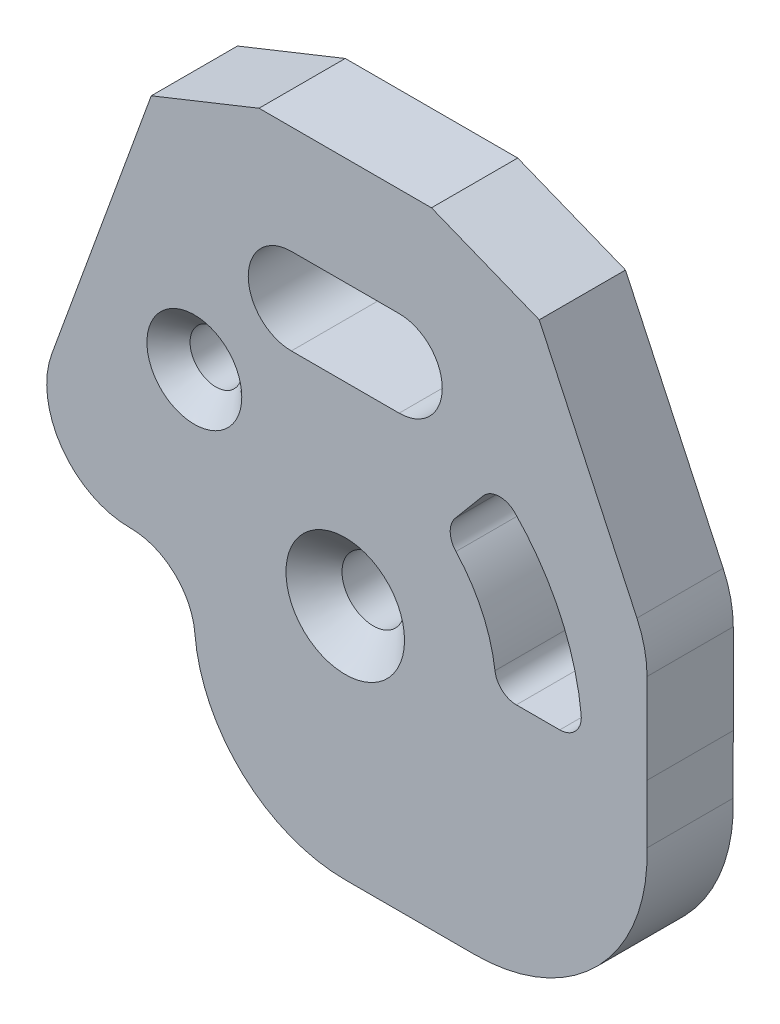
ISO-10303-21;
HEADER;
FILE_DESCRIPTION(('STEP AP214'),'2;1');
FILE_NAME('part.step','',(''),(''),'','','');
FILE_SCHEMA(('AUTOMOTIVE_DESIGN { 1 0 10303 214 1 1 1 1 }'));
ENDSEC;
DATA;
#1=APPLICATION_CONTEXT('core data for automotive mechanical design processes');
#2=APPLICATION_PROTOCOL_DEFINITION('international standard','automotive_design',2000,#1);
#3=PRODUCT_CONTEXT('',#1,'mechanical');
#4=PRODUCT('Part','Part','',(#3));
#5=PRODUCT_RELATED_PRODUCT_CATEGORY('part','',(#4));
#6=PRODUCT_DEFINITION_FORMATION('','',#4);
#7=PRODUCT_DEFINITION_CONTEXT('part definition',#1,'design');
#8=PRODUCT_DEFINITION('design','',#6,#7);
#9=PRODUCT_DEFINITION_SHAPE('','',#8);
#10=(LENGTH_UNIT() NAMED_UNIT(*) SI_UNIT(.MILLI.,.METRE.));
#11=(NAMED_UNIT(*) PLANE_ANGLE_UNIT() SI_UNIT($,.RADIAN.));
#12=(NAMED_UNIT(*) SI_UNIT($,.STERADIAN.) SOLID_ANGLE_UNIT());
#13=UNCERTAINTY_MEASURE_WITH_UNIT(LENGTH_MEASURE(1.E-05),#10,'distance_accuracy_value','');
#14=(GEOMETRIC_REPRESENTATION_CONTEXT(3) GLOBAL_UNCERTAINTY_ASSIGNED_CONTEXT((#13)) GLOBAL_UNIT_ASSIGNED_CONTEXT((#10,
#11,#12)) REPRESENTATION_CONTEXT('',''));
#15=CARTESIAN_POINT('',(0.,0.,0.));
#16=DIRECTION('',(0.,0.,1.));
#17=DIRECTION('',(1.,0.,0.));
#18=AXIS2_PLACEMENT_3D('',#15,#16,#17);
#19=CARTESIAN_POINT('',(-4.,4.47424171782655,4.));
#20=DIRECTION('',(0.371390676354104,-0.928476690885259,0.));
#21=DIRECTION('',(0.928476690885259,0.371390676354104,0.));
#22=AXIS2_PLACEMENT_3D('',#19,#20,#21);
#23=PLANE('',#22);
#24=DIRECTION('',(-0.928476690885259,-0.371390676354104,0.));
#25=VECTOR('',#24,1.);
#26=CARTESIAN_POINT('',(-4.,4.47424171782655,0.));
#27=LINE('',#26,#25);
#28=CARTESIAN_POINT('',(-4.,4.47424171782655,0.));
#29=VERTEX_POINT('',#28);
#30=CARTESIAN_POINT('',(-9.,2.47424171782655,0.));
#31=VERTEX_POINT('',#30);
#32=EDGE_CURVE('E248',#29,#31,#27,.T.);
#33=ORIENTED_EDGE('',*,*,#32,.T.);
#34=DIRECTION('',(0.,0.,-1.));
#35=VECTOR('',#34,1.);
#36=CARTESIAN_POINT('',(-9.,2.47424171782655,4.));
#37=LINE('',#36,#35);
#38=CARTESIAN_POINT('',(-9.,2.47424171782655,4.));
#39=VERTEX_POINT('',#38);
#40=EDGE_CURVE('E11',#39,#31,#37,.T.);
#41=ORIENTED_EDGE('',*,*,#40,.F.);
#42=DIRECTION('',(-0.928476690885259,-0.371390676354104,0.));
#43=VECTOR('',#42,1.);
#44=CARTESIAN_POINT('',(-4.,4.47424171782655,4.));
#45=LINE('',#44,#43);
#46=CARTESIAN_POINT('',(-4.,4.47424171782655,4.));
#47=VERTEX_POINT('',#46);
#48=EDGE_CURVE('E311',#47,#39,#45,.T.);
#49=ORIENTED_EDGE('',*,*,#48,.F.);
#50=DIRECTION('',(0.,0.,-1.));
#51=VECTOR('',#50,1.);
#52=CARTESIAN_POINT('',(-4.,4.47424171782655,4.));
#53=LINE('',#52,#51);
#54=EDGE_CURVE('E343',#47,#29,#53,.T.);
#55=ORIENTED_EDGE('',*,*,#54,.T.);
#56=EDGE_LOOP('',(#33,#41,#49,#55));
#57=FACE_BOUND('',#56,.T.);
#58=ADVANCED_FACE('F39',(#57),#23,.F.);
#59=CARTESIAN_POINT('',(-9.,2.47424171782655,4.));
#60=DIRECTION('',(0.93969262078591,-0.342020143325666,0.));
#61=DIRECTION('',(0.342020143325666,0.93969262078591,0.));
#62=AXIS2_PLACEMENT_3D('',#59,#60,#61);
#63=PLANE('',#62);
#64=DIRECTION('',(-0.342020143325666,-0.93969262078591,0.));
#65=VECTOR('',#64,1.);
#66=CARTESIAN_POINT('',(-9.,2.47424171782655,0.));
#67=LINE('',#66,#65);
#68=CARTESIAN_POINT('',(-13.6164910462462,-10.2094631888496,0.));
#69=VERTEX_POINT('',#68);
#70=EDGE_CURVE('E342',#31,#69,#67,.T.);
#71=ORIENTED_EDGE('',*,*,#70,.T.);
#72=DIRECTION('',(0.,0.,-1.));
#73=VECTOR('',#72,1.);
#74=CARTESIAN_POINT('',(-13.6164910462462,-10.2094631888496,4.));
#75=LINE('',#74,#73);
#76=CARTESIAN_POINT('',(-13.6164910462462,-10.2094631888496,4.));
#77=VERTEX_POINT('',#76);
#78=EDGE_CURVE('E50',#77,#69,#75,.T.);
#79=ORIENTED_EDGE('',*,*,#78,.F.);
#80=DIRECTION('',(-0.342020143325666,-0.93969262078591,0.));
#81=VECTOR('',#80,1.);
#82=CARTESIAN_POINT('',(-9.,2.47424171782655,4.));
#83=LINE('',#82,#81);
#84=EDGE_CURVE('E316',#39,#77,#83,.T.);
#85=ORIENTED_EDGE('',*,*,#84,.F.);
#86=ORIENTED_EDGE('',*,*,#40,.T.);
#87=EDGE_LOOP('',(#71,#79,#85,#86));
#88=FACE_BOUND('',#87,.T.);
#89=ADVANCED_FACE('F439',(#88),#63,.F.);
#90=CARTESIAN_POINT('',(-10.,-11.5257582821734,4.));
#91=DIRECTION('',(0.,0.,-1.));
#92=DIRECTION('',(-1.,0.,0.));
#93=AXIS2_PLACEMENT_3D('',#90,#91,#92);
#94=CYLINDRICAL_SURFACE('',#93,3.84858938577341);
#95=CARTESIAN_POINT('',(-10.,-11.5257582821734,0.));
#96=DIRECTION('',(0.,0.,1.));
#97=DIRECTION('',(1.,0.,0.));
#98=AXIS2_PLACEMENT_3D('',#95,#96,#97);
#99=CIRCLE('',#98,3.84858938577341);
#100=CARTESIAN_POINT('',(-9.97975073778593,-15.3742943970706,0.));
#101=VERTEX_POINT('',#100);
#102=EDGE_CURVE('E347',#69,#101,#99,.T.);
#103=ORIENTED_EDGE('',*,*,#102,.T.);
#104=DIRECTION('',(0.,0.,-1.));
#105=VECTOR('',#104,1.);
#106=CARTESIAN_POINT('',(-9.97975073778593,-15.3742943970706,4.));
#107=LINE('',#106,#105);
#108=CARTESIAN_POINT('',(-9.97975073778593,-15.3742943970706,4.));
#109=VERTEX_POINT('',#108);
#110=EDGE_CURVE('E398',#109,#101,#107,.T.);
#111=ORIENTED_EDGE('',*,*,#110,.F.);
#112=CARTESIAN_POINT('',(-10.,-11.5257582821734,4.));
#113=DIRECTION('',(0.,0.,1.));
#114=DIRECTION('',(1.,0.,0.));
#115=AXIS2_PLACEMENT_3D('',#112,#113,#114);
#116=CIRCLE('',#115,3.84858938577341);
#117=EDGE_CURVE('E317',#77,#109,#116,.T.);
#118=ORIENTED_EDGE('',*,*,#117,.F.);
#119=ORIENTED_EDGE('',*,*,#78,.T.);
#120=EDGE_LOOP('',(#103,#111,#118,#119));
#121=FACE_BOUND('',#120,.T.);
#122=ADVANCED_FACE('F443',(#121),#94,.T.);
#123=CARTESIAN_POINT('',(-9.96396614634065,-18.374283709959,4.));
#124=DIRECTION('',(0.,0.,-1.));
#125=DIRECTION('',(-1.,0.,0.));
#126=AXIS2_PLACEMENT_3D('',#123,#124,#125);
#127=CYLINDRICAL_SURFACE('',#126,3.00003083830351);
#128=CARTESIAN_POINT('',(-9.96396614634065,-18.374283709959,0.));
#129=DIRECTION('',(0.,0.,-1.));
#130=DIRECTION('',(1.,0.,0.));
#131=AXIS2_PLACEMENT_3D('',#128,#129,#130);
#132=CIRCLE('',#131,3.00003083830351);
#133=CARTESIAN_POINT('',(-6.97475479347793,-18.1197242499331,0.));
#134=VERTEX_POINT('',#133);
#135=EDGE_CURVE('E346',#101,#134,#132,.T.);
#136=ORIENTED_EDGE('',*,*,#135,.T.);
#137=DIRECTION('',(0.,0.,-1.));
#138=VECTOR('',#137,1.);
#139=CARTESIAN_POINT('',(-6.97475479347793,-18.1197242499331,4.));
#140=LINE('',#139,#138);
#141=CARTESIAN_POINT('',(-6.97475479347793,-18.1197242499331,4.));
#142=VERTEX_POINT('',#141);
#143=EDGE_CURVE('E391',#142,#134,#140,.T.);
#144=ORIENTED_EDGE('',*,*,#143,.F.);
#145=CARTESIAN_POINT('',(-9.96396614634065,-18.374283709959,4.));
#146=DIRECTION('',(0.,0.,-1.));
#147=DIRECTION('',(1.,0.,0.));
#148=AXIS2_PLACEMENT_3D('',#145,#146,#147);
#149=CIRCLE('',#148,3.00003083830351);
#150=EDGE_CURVE('E321',#109,#142,#149,.T.);
#151=ORIENTED_EDGE('',*,*,#150,.F.);
#152=ORIENTED_EDGE('',*,*,#110,.T.);
#153=EDGE_LOOP('',(#136,#144,#151,#152));
#154=FACE_BOUND('',#153,.T.);
#155=ADVANCED_FACE('F453',(#154),#127,.F.);
#156=CARTESIAN_POINT('',(0.,-17.5257582821734,4.));
#157=DIRECTION('',(0.,0.,-1.));
#158=DIRECTION('',(-1.,0.,0.));
#159=AXIS2_PLACEMENT_3D('',#156,#157,#158);
#160=CYLINDRICAL_SURFACE('',#159,7.);
#161=CARTESIAN_POINT('',(0.,-17.5257582821734,0.));
#162=DIRECTION('',(0.,0.,1.));
#163=DIRECTION('',(1.,0.,0.));
#164=AXIS2_PLACEMENT_3D('',#161,#162,#163);
#165=CIRCLE('',#164,7.);
#166=CARTESIAN_POINT('',(0.,-24.5257582821734,0.));
#167=VERTEX_POINT('',#166);
#168=EDGE_CURVE('E348',#134,#167,#165,.T.);
#169=ORIENTED_EDGE('',*,*,#168,.T.);
#170=DIRECTION('',(0.,0.,-1.));
#171=VECTOR('',#170,1.);
#172=CARTESIAN_POINT('',(0.,-24.5257582821734,4.));
#173=LINE('',#172,#171);
#174=CARTESIAN_POINT('',(0.,-24.5257582821734,4.));
#175=VERTEX_POINT('',#174);
#176=EDGE_CURVE('E388',#175,#167,#173,.T.);
#177=ORIENTED_EDGE('',*,*,#176,.F.);
#178=CARTESIAN_POINT('',(0.,-17.5257582821734,4.));
#179=DIRECTION('',(0.,0.,1.));
#180=DIRECTION('',(1.,0.,0.));
#181=AXIS2_PLACEMENT_3D('',#178,#179,#180);
#182=CIRCLE('',#181,7.);
#183=EDGE_CURVE('E323',#142,#175,#182,.T.);
#184=ORIENTED_EDGE('',*,*,#183,.F.);
#185=ORIENTED_EDGE('',*,*,#143,.T.);
#186=EDGE_LOOP('',(#169,#177,#184,#185));
#187=FACE_BOUND('',#186,.T.);
#188=ADVANCED_FACE('F454',(#187),#160,.T.);
#189=CARTESIAN_POINT('',(0.,-24.5257582821734,4.));
#190=DIRECTION('',(0.,1.,0.));
#191=DIRECTION('',(-1.,0.,0.));
#192=AXIS2_PLACEMENT_3D('',#189,#190,#191);
#193=PLANE('',#192);
#194=DIRECTION('',(1.,0.,0.));
#195=VECTOR('',#194,1.);
#196=CARTESIAN_POINT('',(0.,-24.5257582821734,0.));
#197=LINE('',#196,#195);
#198=CARTESIAN_POINT('',(6.,-24.5257582821734,0.));
#199=VERTEX_POINT('',#198);
#200=EDGE_CURVE('E355',#167,#199,#197,.T.);
#201=ORIENTED_EDGE('',*,*,#200,.T.);
#202=DIRECTION('',(0.,0.,-1.));
#203=VECTOR('',#202,1.);
#204=CARTESIAN_POINT('',(6.,-24.5257582821734,4.));
#205=LINE('',#204,#203);
#206=CARTESIAN_POINT('',(6.,-24.5257582821734,4.));
#207=VERTEX_POINT('',#206);
#208=EDGE_CURVE('E390',#207,#199,#205,.T.);
#209=ORIENTED_EDGE('',*,*,#208,.F.);
#210=DIRECTION('',(1.,0.,0.));
#211=VECTOR('',#210,1.);
#212=CARTESIAN_POINT('',(0.,-24.5257582821734,4.));
#213=LINE('',#212,#211);
#214=EDGE_CURVE('E324',#175,#207,#213,.T.);
#215=ORIENTED_EDGE('',*,*,#214,.F.);
#216=ORIENTED_EDGE('',*,*,#176,.T.);
#217=EDGE_LOOP('',(#201,#209,#215,#216));
#218=FACE_BOUND('',#217,.T.);
#219=ADVANCED_FACE('F458',(#218),#193,.F.);
#220=CARTESIAN_POINT('',(6.,-16.5257582821734,4.));
#221=DIRECTION('',(0.,0.,-1.));
#222=DIRECTION('',(-1.,0.,0.));
#223=AXIS2_PLACEMENT_3D('',#220,#221,#222);
#224=CYLINDRICAL_SURFACE('',#223,8.);
#225=CARTESIAN_POINT('',(6.,-16.5257582821734,0.));
#226=DIRECTION('',(0.,0.,1.));
#227=DIRECTION('',(-1.,0.,0.));
#228=AXIS2_PLACEMENT_3D('',#225,#226,#227);
#229=CIRCLE('',#228,8.);
#230=CARTESIAN_POINT('',(13.9951489566235,-16.2472027914667,0.));
#231=VERTEX_POINT('',#230);
#232=EDGE_CURVE('E352',#199,#231,#229,.T.);
#233=ORIENTED_EDGE('',*,*,#232,.T.);
#234=DIRECTION('',(0.,0.,-1.));
#235=VECTOR('',#234,1.);
#236=CARTESIAN_POINT('',(13.9951489566235,-16.2472027914667,4.));
#237=LINE('',#236,#235);
#238=CARTESIAN_POINT('',(13.9951489566235,-16.2472027914667,4.));
#239=VERTEX_POINT('',#238);
#240=EDGE_CURVE('E383',#239,#231,#237,.T.);
#241=ORIENTED_EDGE('',*,*,#240,.F.);
#242=CARTESIAN_POINT('',(6.,-16.5257582821734,4.));
#243=DIRECTION('',(0.,0.,1.));
#244=DIRECTION('',(-1.,0.,0.));
#245=AXIS2_PLACEMENT_3D('',#242,#243,#244);
#246=CIRCLE('',#245,8.);
#247=EDGE_CURVE('E330',#207,#239,#246,.T.);
#248=ORIENTED_EDGE('',*,*,#247,.F.);
#249=ORIENTED_EDGE('',*,*,#208,.T.);
#250=EDGE_LOOP('',(#233,#241,#248,#249));
#251=FACE_BOUND('',#250,.T.);
#252=ADVANCED_FACE('F468',(#251),#224,.T.);
#253=CARTESIAN_POINT('',(14.,-13.5257582821734,4.));
#254=DIRECTION('',(-0.999998411305769,0.00178252235280163,0.));
#255=DIRECTION('',(-0.00178252235280163,-0.999998411305769,0.));
#256=AXIS2_PLACEMENT_3D('',#253,#254,#255);
#257=PLANE('',#256);
#258=DIRECTION('',(0.00178252235280163,0.999998411305769,0.));
#259=VECTOR('',#258,1.);
#260=CARTESIAN_POINT('',(14.,-13.5257582821734,0.));
#261=LINE('',#260,#259);
#262=CARTESIAN_POINT('',(14.,-13.5257582821734,0.));
#263=VERTEX_POINT('',#262);
#264=EDGE_CURVE('E358',#231,#263,#261,.T.);
#265=ORIENTED_EDGE('',*,*,#264,.T.);
#266=DIRECTION('',(0.,0.,-1.));
#267=VECTOR('',#266,1.);
#268=CARTESIAN_POINT('',(14.,-13.5257582821734,4.));
#269=LINE('',#268,#267);
#270=CARTESIAN_POINT('',(14.,-13.5257582821734,4.));
#271=VERTEX_POINT('',#270);
#272=EDGE_CURVE('E381',#271,#263,#269,.T.);
#273=ORIENTED_EDGE('',*,*,#272,.F.);
#274=DIRECTION('',(0.00178252235280163,0.999998411305769,0.));
#275=VECTOR('',#274,1.);
#276=CARTESIAN_POINT('',(14.,-13.5257582821734,4.));
#277=LINE('',#276,#275);
#278=EDGE_CURVE('E328',#239,#271,#277,.T.);
#279=ORIENTED_EDGE('',*,*,#278,.F.);
#280=ORIENTED_EDGE('',*,*,#240,.T.);
#281=EDGE_LOOP('',(#265,#273,#279,#280));
#282=FACE_BOUND('',#281,.T.);
#283=ADVANCED_FACE('F469',(#282),#257,.F.);
#284=CARTESIAN_POINT('',(14.,-9.356766197936,4.));
#285=DIRECTION('',(-1.,0.,0.));
#286=DIRECTION('',(0.,0.,1.));
#287=AXIS2_PLACEMENT_3D('',#284,#285,#286);
#288=PLANE('',#287);
#289=DIRECTION('',(0.,1.,0.));
#290=VECTOR('',#289,1.);
#291=CARTESIAN_POINT('',(14.,-9.356766197936,0.));
#292=LINE('',#291,#290);
#293=CARTESIAN_POINT('',(14.,-9.356766197936,0.));
#294=VERTEX_POINT('',#293);
#295=EDGE_CURVE('E356',#263,#294,#292,.T.);
#296=ORIENTED_EDGE('',*,*,#295,.T.);
#297=DIRECTION('',(0.,0.,-1.));
#298=VECTOR('',#297,1.);
#299=CARTESIAN_POINT('',(14.,-9.356766197936,4.));
#300=LINE('',#299,#298);
#301=CARTESIAN_POINT('',(14.,-9.356766197936,4.));
#302=VERTEX_POINT('',#301);
#303=EDGE_CURVE('E378',#302,#294,#300,.T.);
#304=ORIENTED_EDGE('',*,*,#303,.F.);
#305=DIRECTION('',(0.,1.,0.));
#306=VECTOR('',#305,1.);
#307=CARTESIAN_POINT('',(14.,-9.356766197936,4.));
#308=LINE('',#307,#306);
#309=EDGE_CURVE('E332',#271,#302,#308,.T.);
#310=ORIENTED_EDGE('',*,*,#309,.F.);
#311=ORIENTED_EDGE('',*,*,#272,.T.);
#312=EDGE_LOOP('',(#296,#304,#310,#311));
#313=FACE_BOUND('',#312,.T.);
#314=ADVANCED_FACE('F474',(#313),#288,.F.);
#315=CARTESIAN_POINT('',(9.,-9.356766197936,4.));
#316=DIRECTION('',(0.,0.,-1.));
#317=DIRECTION('',(-1.,0.,0.));
#318=AXIS2_PLACEMENT_3D('',#315,#316,#317);
#319=CYLINDRICAL_SURFACE('',#318,5.);
#320=CARTESIAN_POINT('',(9.,-9.356766197936,0.));
#321=DIRECTION('',(0.,0.,1.));
#322=DIRECTION('',(-1.,0.,0.));
#323=AXIS2_PLACEMENT_3D('',#320,#321,#322);
#324=CIRCLE('',#323,5.);
#325=CARTESIAN_POINT('',(13.5315389351833,-7.24367488923252,0.));
#326=VERTEX_POINT('',#325);
#327=EDGE_CURVE('E359',#294,#326,#324,.T.);
#328=ORIENTED_EDGE('',*,*,#327,.T.);
#329=DIRECTION('',(0.,0.,-1.));
#330=VECTOR('',#329,1.);
#331=CARTESIAN_POINT('',(13.5315389351833,-7.24367488923252,4.));
#332=LINE('',#331,#330);
#333=CARTESIAN_POINT('',(13.5315389351833,-7.24367488923252,4.));
#334=VERTEX_POINT('',#333);
#335=EDGE_CURVE('E374',#334,#326,#332,.T.);
#336=ORIENTED_EDGE('',*,*,#335,.F.);
#337=CARTESIAN_POINT('',(9.,-9.356766197936,4.));
#338=DIRECTION('',(0.,0.,1.));
#339=DIRECTION('',(-1.,0.,0.));
#340=AXIS2_PLACEMENT_3D('',#337,#338,#339);
#341=CIRCLE('',#340,5.);
#342=EDGE_CURVE('E334',#302,#334,#341,.T.);
#343=ORIENTED_EDGE('',*,*,#342,.F.);
#344=ORIENTED_EDGE('',*,*,#303,.T.);
#345=EDGE_LOOP('',(#328,#336,#343,#344));
#346=FACE_BOUND('',#345,.T.);
#347=ADVANCED_FACE('F481',(#346),#319,.T.);
#348=CARTESIAN_POINT('',(9.,2.47424171782655,4.));
#349=DIRECTION('',(-0.906307787036651,-0.422618261740697,0.));
#350=DIRECTION('',(0.422618261740697,-0.906307787036651,0.));
#351=AXIS2_PLACEMENT_3D('',#348,#349,#350);
#352=PLANE('',#351);
#353=DIRECTION('',(-0.422618261740697,0.906307787036651,0.));
#354=VECTOR('',#353,1.);
#355=CARTESIAN_POINT('',(9.,2.47424171782655,0.));
#356=LINE('',#355,#354);
#357=CARTESIAN_POINT('',(9.,2.47424171782655,0.));
#358=VERTEX_POINT('',#357);
#359=EDGE_CURVE('E362',#326,#358,#356,.T.);
#360=ORIENTED_EDGE('',*,*,#359,.T.);
#361=DIRECTION('',(0.,0.,-1.));
#362=VECTOR('',#361,1.);
#363=CARTESIAN_POINT('',(9.,2.47424171782655,4.));
#364=LINE('',#363,#362);
#365=CARTESIAN_POINT('',(9.,2.47424171782655,4.));
#366=VERTEX_POINT('',#365);
#367=EDGE_CURVE('E375',#366,#358,#364,.T.);
#368=ORIENTED_EDGE('',*,*,#367,.F.);
#369=DIRECTION('',(-0.422618261740697,0.906307787036651,0.));
#370=VECTOR('',#369,1.);
#371=CARTESIAN_POINT('',(9.,2.47424171782655,4.));
#372=LINE('',#371,#370);
#373=EDGE_CURVE('E333',#334,#366,#372,.T.);
#374=ORIENTED_EDGE('',*,*,#373,.F.);
#375=ORIENTED_EDGE('',*,*,#335,.T.);
#376=EDGE_LOOP('',(#360,#368,#374,#375));
#377=FACE_BOUND('',#376,.T.);
#378=ADVANCED_FACE('F484',(#377),#352,.F.);
#379=CARTESIAN_POINT('',(4.,4.47424171782655,4.));
#380=DIRECTION('',(-0.371390676354104,-0.928476690885259,0.));
#381=DIRECTION('',(0.928476690885259,-0.371390676354104,0.));
#382=AXIS2_PLACEMENT_3D('',#379,#380,#381);
#383=PLANE('',#382);
#384=DIRECTION('',(-0.928476690885259,0.371390676354104,0.));
#385=VECTOR('',#384,1.);
#386=CARTESIAN_POINT('',(4.,4.47424171782655,0.));
#387=LINE('',#386,#385);
#388=CARTESIAN_POINT('',(4.,4.47424171782655,0.));
#389=VERTEX_POINT('',#388);
#390=EDGE_CURVE('E365',#358,#389,#387,.T.);
#391=ORIENTED_EDGE('',*,*,#390,.T.);
#392=DIRECTION('',(0.,0.,-1.));
#393=VECTOR('',#392,1.);
#394=CARTESIAN_POINT('',(4.,4.47424171782655,4.));
#395=LINE('',#394,#393);
#396=CARTESIAN_POINT('',(4.,4.47424171782655,4.));
#397=VERTEX_POINT('',#396);
#398=EDGE_CURVE('E369',#397,#389,#395,.T.);
#399=ORIENTED_EDGE('',*,*,#398,.F.);
#400=DIRECTION('',(-0.928476690885259,0.371390676354104,0.));
#401=VECTOR('',#400,1.);
#402=CARTESIAN_POINT('',(4.,4.47424171782655,4.));
#403=LINE('',#402,#401);
#404=EDGE_CURVE('E340',#366,#397,#403,.T.);
#405=ORIENTED_EDGE('',*,*,#404,.F.);
#406=ORIENTED_EDGE('',*,*,#367,.T.);
#407=EDGE_LOOP('',(#391,#399,#405,#406));
#408=FACE_BOUND('',#407,.T.);
#409=ADVANCED_FACE('F489',(#408),#383,.F.);
#410=CARTESIAN_POINT('',(4.,4.47424171782655,4.));
#411=DIRECTION('',(0.,-1.,0.));
#412=DIRECTION('',(1.,0.,0.));
#413=AXIS2_PLACEMENT_3D('',#410,#411,#412);
#414=PLANE('',#413);
#415=DIRECTION('',(-1.,0.,0.));
#416=VECTOR('',#415,1.);
#417=CARTESIAN_POINT('',(4.,4.47424171782655,0.));
#418=LINE('',#417,#416);
#419=EDGE_CURVE('E320',#389,#29,#418,.T.);
#420=ORIENTED_EDGE('',*,*,#419,.T.);
#421=ORIENTED_EDGE('',*,*,#54,.F.);
#422=DIRECTION('',(-1.,0.,0.));
#423=VECTOR('',#422,1.);
#424=CARTESIAN_POINT('',(4.,4.47424171782655,4.));
#425=LINE('',#424,#423);
#426=EDGE_CURVE('E337',#397,#47,#425,.T.);
#427=ORIENTED_EDGE('',*,*,#426,.F.);
#428=ORIENTED_EDGE('',*,*,#398,.T.);
#429=EDGE_LOOP('',(#420,#421,#427,#428));
#430=FACE_BOUND('',#429,.T.);
#431=ADVANCED_FACE('F424',(#430),#414,.F.);
#432=CARTESIAN_POINT('',(-10.,-11.5257582821734,4.));
#433=DIRECTION('',(0.,0.,1.));
#434=DIRECTION('',(1.,0.,0.));
#435=AXIS2_PLACEMENT_3D('',#432,#433,#434);
#436=PLANE('',#435);
#437=CARTESIAN_POINT('',(-7.,-7.52575828217345,4.));
#438=DIRECTION('',(0.,0.,1.));
#439=DIRECTION('',(1.,0.,0.));
#440=AXIS2_PLACEMENT_3D('',#437,#438,#439);
#441=CIRCLE('',#440,2.2);
#442=CARTESIAN_POINT('',(-4.8,-7.52575828217345,4.));
#443=VERTEX_POINT('',#442);
#444=EDGE_CURVE('E414',#443,#443,#441,.T.);
#445=ORIENTED_EDGE('',*,*,#444,.F.);
#446=EDGE_LOOP('',(#445));
#447=FACE_BOUND('',#446,.T.);
#448=CARTESIAN_POINT('',(0.,-13.5257582821735,4.));
#449=DIRECTION('',(0.,0.,1.));
#450=DIRECTION('',(1.,0.,0.));
#451=AXIS2_PLACEMENT_3D('',#448,#449,#450);
#452=CIRCLE('',#451,2.75);
#453=CARTESIAN_POINT('',(2.75,-13.5257582821735,4.));
#454=VERTEX_POINT('',#453);
#455=EDGE_CURVE('E404',#454,#454,#452,.T.);
#456=ORIENTED_EDGE('',*,*,#455,.F.);
#457=EDGE_LOOP('',(#456));
#458=FACE_BOUND('',#457,.T.);
#459=CARTESIAN_POINT('',(-2.5,-2.52575828217345,4.));
#460=DIRECTION('',(0.,0.,1.));
#461=DIRECTION('',(1.,0.,0.));
#462=AXIS2_PLACEMENT_3D('',#459,#460,#461);
#463=CIRCLE('',#462,2.);
#464=CARTESIAN_POINT('',(-2.5,-0.525758282173447,4.));
#465=VERTEX_POINT('',#464);
#466=CARTESIAN_POINT('',(-2.5,-4.52575828217345,4.));
#467=VERTEX_POINT('',#466);
#468=EDGE_CURVE('E54',#465,#467,#463,.T.);
#469=ORIENTED_EDGE('',*,*,#468,.F.);
#470=DIRECTION('',(-1.,0.,0.));
#471=VECTOR('',#470,1.);
#472=CARTESIAN_POINT('',(-2.5,-0.525758282173447,4.));
#473=LINE('',#472,#471);
#474=CARTESIAN_POINT('',(2.5,-0.525758282173446,4.));
#475=VERTEX_POINT('',#474);
#476=EDGE_CURVE('E226',#475,#465,#473,.T.);
#477=ORIENTED_EDGE('',*,*,#476,.F.);
#478=CARTESIAN_POINT('',(2.5,-2.52575828217345,4.));
#479=DIRECTION('',(0.,0.,1.));
#480=DIRECTION('',(1.,0.,0.));
#481=AXIS2_PLACEMENT_3D('',#478,#479,#480);
#482=CIRCLE('',#481,2.);
#483=CARTESIAN_POINT('',(2.5,-4.52575828217345,4.));
#484=VERTEX_POINT('',#483);
#485=EDGE_CURVE('E233',#484,#475,#482,.T.);
#486=ORIENTED_EDGE('',*,*,#485,.F.);
#487=DIRECTION('',(1.,0.,0.));
#488=VECTOR('',#487,1.);
#489=CARTESIAN_POINT('',(-2.5,-4.52575828217345,4.));
#490=LINE('',#489,#488);
#491=EDGE_CURVE('E238',#467,#484,#490,.T.);
#492=ORIENTED_EDGE('',*,*,#491,.F.);
#493=EDGE_LOOP('',(#469,#477,#486,#492));
#494=FACE_BOUND('',#493,.T.);
#495=CARTESIAN_POINT('',(9.9498743710662,-12.5257582821734,4.));
#496=DIRECTION('',(0.,0.,1.));
#497=DIRECTION('',(1.,0.,0.));
#498=AXIS2_PLACEMENT_3D('',#495,#496,#497);
#499=CIRCLE('',#498,1.);
#500=CARTESIAN_POINT('',(9.9498743710662,-13.5257582821734,4.));
#501=VERTEX_POINT('',#500);
#502=CARTESIAN_POINT('',(10.9448618081728,-12.4257582821734,4.));
#503=VERTEX_POINT('',#502);
#504=EDGE_CURVE('E61',#501,#503,#499,.T.);
#505=ORIENTED_EDGE('',*,*,#504,.F.);
#506=DIRECTION('',(1.,0.,0.));
#507=VECTOR('',#506,1.);
#508=CARTESIAN_POINT('',(7.93725393319377,-13.5257582821734,4.));
#509=LINE('',#508,#507);
#510=CARTESIAN_POINT('',(7.93725393319377,-13.5257582821734,4.));
#511=VERTEX_POINT('',#510);
#512=EDGE_CURVE('E268',#511,#501,#509,.T.);
#513=ORIENTED_EDGE('',*,*,#512,.F.);
#514=CARTESIAN_POINT('',(7.93725393319377,-12.5257582821734,4.));
#515=DIRECTION('',(0.,0.,1.));
#516=DIRECTION('',(-1.,0.,0.));
#517=AXIS2_PLACEMENT_3D('',#514,#515,#516);
#518=CIRCLE('',#517,1.);
#519=CARTESIAN_POINT('',(6.94509719154455,-12.6507582821734,4.));
#520=VERTEX_POINT('',#519);
#521=EDGE_CURVE('E271',#520,#511,#518,.T.);
#522=ORIENTED_EDGE('',*,*,#521,.F.);
#523=CARTESIAN_POINT('',(0.,-13.5257582821734,4.));
#524=DIRECTION('',(0.,0.,-1.));
#525=DIRECTION('',(1.,0.,0.));
#526=AXIS2_PLACEMENT_3D('',#523,#524,#525);
#527=CIRCLE('',#526,7.);
#528=CARTESIAN_POINT('',(5.13451131052272,-8.76794433014524,4.));
#529=VERTEX_POINT('',#528);
#530=EDGE_CURVE('E274',#529,#520,#527,.T.);
#531=ORIENTED_EDGE('',*,*,#530,.F.);
#532=CARTESIAN_POINT('',(5.86801292631167,-8.08825662271264,4.));
#533=DIRECTION('',(0.,0.,1.));
#534=DIRECTION('',(1.,0.,0.));
#535=AXIS2_PLACEMENT_3D('',#532,#533,#534);
#536=CIRCLE('',#535,0.999999999999999);
#537=CARTESIAN_POINT('',(5.10196848319269,-7.4454690130261,4.));
#538=VERTEX_POINT('',#537);
#539=EDGE_CURVE('E279',#538,#529,#536,.T.);
#540=ORIENTED_EDGE('',*,*,#539,.F.);
#541=DIRECTION('',(-0.642787609686538,-0.766044443118979,0.));
#542=VECTOR('',#541,1.);
#543=CARTESIAN_POINT('',(5.10196848319269,-7.4454690130261,4.));
#544=LINE('',#543,#542);
#545=CARTESIAN_POINT('',(6.39565596365899,-5.90371231048624,4.));
#546=VERTEX_POINT('',#545);
#547=EDGE_CURVE('E283',#546,#538,#544,.T.);
#548=ORIENTED_EDGE('',*,*,#547,.F.);
#549=CARTESIAN_POINT('',(7.16170040677796,-6.54649992017278,4.));
#550=DIRECTION('',(0.,0.,1.));
#551=DIRECTION('',(-1.,0.,0.));
#552=AXIS2_PLACEMENT_3D('',#549,#550,#551);
#553=CIRCLE('',#552,1.);
#554=CARTESIAN_POINT('',(7.87787044745576,-5.84857408397271,4.));
#555=VERTEX_POINT('',#554);
#556=EDGE_CURVE('E282',#555,#546,#553,.T.);
#557=ORIENTED_EDGE('',*,*,#556,.F.);
#558=CARTESIAN_POINT('',(0.,-13.5257582821734,4.));
#559=DIRECTION('',(0.,0.,1.));
#560=DIRECTION('',(1.,0.,0.));
#561=AXIS2_PLACEMENT_3D('',#558,#559,#560);
#562=CIRCLE('',#561,11.);
#563=EDGE_CURVE('E290',#503,#555,#562,.T.);
#564=ORIENTED_EDGE('',*,*,#563,.F.);
#565=EDGE_LOOP('',(#505,#513,#522,#531,#540,#548,#557,#564));
#566=FACE_BOUND('',#565,.T.);
#567=ORIENTED_EDGE('',*,*,#48,.T.);
#568=ORIENTED_EDGE('',*,*,#84,.T.);
#569=ORIENTED_EDGE('',*,*,#117,.T.);
#570=ORIENTED_EDGE('',*,*,#150,.T.);
#571=ORIENTED_EDGE('',*,*,#183,.T.);
#572=ORIENTED_EDGE('',*,*,#214,.T.);
#573=ORIENTED_EDGE('',*,*,#247,.T.);
#574=ORIENTED_EDGE('',*,*,#278,.T.);
#575=ORIENTED_EDGE('',*,*,#309,.T.);
#576=ORIENTED_EDGE('',*,*,#342,.T.);
#577=ORIENTED_EDGE('',*,*,#373,.T.);
#578=ORIENTED_EDGE('',*,*,#404,.T.);
#579=ORIENTED_EDGE('',*,*,#426,.T.);
#580=EDGE_LOOP('',(#567,#568,#569,#570,#571,#572,#573,#574,#575,#576,#577,#578,#579));
#581=FACE_BOUND('',#580,.T.);
#582=ADVANCED_FACE('F423',(#447,#458,#494,#566,#581),#436,.T.);
#583=CARTESIAN_POINT('',(-10.,-11.5257582821734,0.));
#584=DIRECTION('',(0.,0.,1.));
#585=DIRECTION('',(1.,0.,0.));
#586=AXIS2_PLACEMENT_3D('',#583,#584,#585);
#587=PLANE('',#586);
#588=CARTESIAN_POINT('',(-7.,-7.52575828217345,0.));
#589=DIRECTION('',(0.,0.,1.));
#590=DIRECTION('',(1.,0.,0.));
#591=AXIS2_PLACEMENT_3D('',#588,#589,#590);
#592=CIRCLE('',#591,1.19999999999999);
#593=CARTESIAN_POINT('',(-5.8,-7.52575828217345,0.));
#594=VERTEX_POINT('',#593);
#595=EDGE_CURVE('E45',#594,#594,#592,.T.);
#596=ORIENTED_EDGE('',*,*,#595,.T.);
#597=EDGE_LOOP('',(#596));
#598=FACE_BOUND('',#597,.T.);
#599=CARTESIAN_POINT('',(0.,-13.5257582821735,0.));
#600=DIRECTION('',(0.,0.,1.));
#601=DIRECTION('',(1.,0.,0.));
#602=AXIS2_PLACEMENT_3D('',#599,#600,#601);
#603=CIRCLE('',#602,1.44999999999999);
#604=CARTESIAN_POINT('',(1.45,-13.5257582821735,0.));
#605=VERTEX_POINT('',#604);
#606=EDGE_CURVE('E270',#605,#605,#603,.T.);
#607=ORIENTED_EDGE('',*,*,#606,.T.);
#608=EDGE_LOOP('',(#607));
#609=FACE_BOUND('',#608,.T.);
#610=DIRECTION('',(-1.,0.,0.));
#611=VECTOR('',#610,1.);
#612=CARTESIAN_POINT('',(-2.5,-0.525758282173447,0.));
#613=LINE('',#612,#611);
#614=CARTESIAN_POINT('',(2.5,-0.525758282173446,0.));
#615=VERTEX_POINT('',#614);
#616=CARTESIAN_POINT('',(-2.5,-0.525758282173447,0.));
#617=VERTEX_POINT('',#616);
#618=EDGE_CURVE('E214',#615,#617,#613,.T.);
#619=ORIENTED_EDGE('',*,*,#618,.T.);
#620=CARTESIAN_POINT('',(-2.5,-2.52575828217345,0.));
#621=DIRECTION('',(0.,0.,1.));
#622=DIRECTION('',(1.,0.,0.));
#623=AXIS2_PLACEMENT_3D('',#620,#621,#622);
#624=CIRCLE('',#623,2.);
#625=CARTESIAN_POINT('',(-2.5,-4.52575828217345,0.));
#626=VERTEX_POINT('',#625);
#627=EDGE_CURVE('E207',#617,#626,#624,.T.);
#628=ORIENTED_EDGE('',*,*,#627,.T.);
#629=DIRECTION('',(1.,0.,0.));
#630=VECTOR('',#629,1.);
#631=CARTESIAN_POINT('',(-2.5,-4.52575828217345,0.));
#632=LINE('',#631,#630);
#633=CARTESIAN_POINT('',(2.5,-4.52575828217345,0.));
#634=VERTEX_POINT('',#633);
#635=EDGE_CURVE('E218',#626,#634,#632,.T.);
#636=ORIENTED_EDGE('',*,*,#635,.T.);
#637=CARTESIAN_POINT('',(2.5,-2.52575828217345,0.));
#638=DIRECTION('',(0.,0.,1.));
#639=DIRECTION('',(1.,0.,0.));
#640=AXIS2_PLACEMENT_3D('',#637,#638,#639);
#641=CIRCLE('',#640,2.);
#642=EDGE_CURVE('E224',#634,#615,#641,.T.);
#643=ORIENTED_EDGE('',*,*,#642,.T.);
#644=EDGE_LOOP('',(#619,#628,#636,#643));
#645=FACE_BOUND('',#644,.T.);
#646=DIRECTION('',(1.,0.,0.));
#647=VECTOR('',#646,1.);
#648=CARTESIAN_POINT('',(7.93725393319377,-13.5257582821734,0.));
#649=LINE('',#648,#647);
#650=CARTESIAN_POINT('',(7.93725393319377,-13.5257582821734,0.));
#651=VERTEX_POINT('',#650);
#652=CARTESIAN_POINT('',(9.9498743710662,-13.5257582821734,0.));
#653=VERTEX_POINT('',#652);
#654=EDGE_CURVE('E252',#651,#653,#649,.T.);
#655=ORIENTED_EDGE('',*,*,#654,.T.);
#656=CARTESIAN_POINT('',(9.9498743710662,-12.5257582821734,0.));
#657=DIRECTION('',(0.,0.,1.));
#658=DIRECTION('',(1.,0.,0.));
#659=AXIS2_PLACEMENT_3D('',#656,#657,#658);
#660=CIRCLE('',#659,1.);
#661=CARTESIAN_POINT('',(10.9448618081728,-12.4257582821734,0.));
#662=VERTEX_POINT('',#661);
#663=EDGE_CURVE('E275',#653,#662,#660,.T.);
#664=ORIENTED_EDGE('',*,*,#663,.T.);
#665=CARTESIAN_POINT('',(0.,-13.5257582821734,0.));
#666=DIRECTION('',(0.,0.,1.));
#667=DIRECTION('',(1.,0.,0.));
#668=AXIS2_PLACEMENT_3D('',#665,#666,#667);
#669=CIRCLE('',#668,11.);
#670=CARTESIAN_POINT('',(7.87787044745576,-5.84857408397271,0.));
#671=VERTEX_POINT('',#670);
#672=EDGE_CURVE('E306',#662,#671,#669,.T.);
#673=ORIENTED_EDGE('',*,*,#672,.T.);
#674=CARTESIAN_POINT('',(7.16170040677796,-6.54649992017278,0.));
#675=DIRECTION('',(0.,0.,1.));
#676=DIRECTION('',(-1.,0.,0.));
#677=AXIS2_PLACEMENT_3D('',#674,#675,#676);
#678=CIRCLE('',#677,1.);
#679=CARTESIAN_POINT('',(6.39565596365899,-5.90371231048624,0.));
#680=VERTEX_POINT('',#679);
#681=EDGE_CURVE('E304',#671,#680,#678,.T.);
#682=ORIENTED_EDGE('',*,*,#681,.T.);
#683=DIRECTION('',(-0.642787609686538,-0.766044443118979,0.));
#684=VECTOR('',#683,1.);
#685=CARTESIAN_POINT('',(5.10196848319269,-7.4454690130261,0.));
#686=LINE('',#685,#684);
#687=CARTESIAN_POINT('',(5.10196848319269,-7.4454690130261,0.));
#688=VERTEX_POINT('',#687);
#689=EDGE_CURVE('E305',#680,#688,#686,.T.);
#690=ORIENTED_EDGE('',*,*,#689,.T.);
#691=CARTESIAN_POINT('',(5.86801292631167,-8.08825662271264,0.));
#692=DIRECTION('',(0.,0.,1.));
#693=DIRECTION('',(1.,0.,0.));
#694=AXIS2_PLACEMENT_3D('',#691,#692,#693);
#695=CIRCLE('',#694,0.999999999999999);
#696=CARTESIAN_POINT('',(5.13451131052272,-8.76794433014524,0.));
#697=VERTEX_POINT('',#696);
#698=EDGE_CURVE('E297',#688,#697,#695,.T.);
#699=ORIENTED_EDGE('',*,*,#698,.T.);
#700=CARTESIAN_POINT('',(0.,-13.5257582821734,0.));
#701=DIRECTION('',(0.,0.,-1.));
#702=DIRECTION('',(1.,0.,0.));
#703=AXIS2_PLACEMENT_3D('',#700,#701,#702);
#704=CIRCLE('',#703,7.);
#705=CARTESIAN_POINT('',(6.94509719154455,-12.6507582821734,0.));
#706=VERTEX_POINT('',#705);
#707=EDGE_CURVE('E298',#697,#706,#704,.T.);
#708=ORIENTED_EDGE('',*,*,#707,.T.);
#709=CARTESIAN_POINT('',(7.93725393319377,-12.5257582821734,0.));
#710=DIRECTION('',(0.,0.,1.));
#711=DIRECTION('',(-1.,0.,0.));
#712=AXIS2_PLACEMENT_3D('',#709,#710,#711);
#713=CIRCLE('',#712,1.);
#714=EDGE_CURVE('E291',#706,#651,#713,.T.);
#715=ORIENTED_EDGE('',*,*,#714,.T.);
#716=EDGE_LOOP('',(#655,#664,#673,#682,#690,#699,#708,#715));
#717=FACE_BOUND('',#716,.T.);
#718=ORIENTED_EDGE('',*,*,#32,.F.);
#719=ORIENTED_EDGE('',*,*,#419,.F.);
#720=ORIENTED_EDGE('',*,*,#390,.F.);
#721=ORIENTED_EDGE('',*,*,#359,.F.);
#722=ORIENTED_EDGE('',*,*,#327,.F.);
#723=ORIENTED_EDGE('',*,*,#295,.F.);
#724=ORIENTED_EDGE('',*,*,#264,.F.);
#725=ORIENTED_EDGE('',*,*,#232,.F.);
#726=ORIENTED_EDGE('',*,*,#200,.F.);
#727=ORIENTED_EDGE('',*,*,#168,.F.);
#728=ORIENTED_EDGE('',*,*,#135,.F.);
#729=ORIENTED_EDGE('',*,*,#102,.F.);
#730=ORIENTED_EDGE('',*,*,#70,.F.);
#731=EDGE_LOOP('',(#718,#719,#720,#721,#722,#723,#724,#725,#726,#727,#728,#729,#730));
#732=FACE_BOUND('',#731,.T.);
#733=ADVANCED_FACE('F223',(#598,#609,#645,#717,#732),#587,.F.);
#734=CARTESIAN_POINT('',(9.9498743710662,-12.5257582821734,0.));
#735=DIRECTION('',(0.,0.,1.));
#736=DIRECTION('',(1.,0.,0.));
#737=AXIS2_PLACEMENT_3D('',#734,#735,#736);
#738=CYLINDRICAL_SURFACE('',#737,1.);
#739=ORIENTED_EDGE('',*,*,#504,.T.);
#740=DIRECTION('',(0.,0.,1.));
#741=VECTOR('',#740,1.);
#742=CARTESIAN_POINT('',(10.9448618081728,-12.4257582821734,0.));
#743=LINE('',#742,#741);
#744=EDGE_CURVE('E249',#662,#503,#743,.T.);
#745=ORIENTED_EDGE('',*,*,#744,.F.);
#746=ORIENTED_EDGE('',*,*,#663,.F.);
#747=DIRECTION('',(0.,0.,1.));
#748=VECTOR('',#747,1.);
#749=CARTESIAN_POINT('',(9.9498743710662,-13.5257582821734,0.));
#750=LINE('',#749,#748);
#751=EDGE_CURVE('E264',#653,#501,#750,.T.);
#752=ORIENTED_EDGE('',*,*,#751,.T.);
#753=EDGE_LOOP('',(#739,#745,#746,#752));
#754=FACE_BOUND('',#753,.T.);
#755=ADVANCED_FACE('F494',(#754),#738,.F.);
#756=CARTESIAN_POINT('',(7.93725393319377,-13.5257582821734,0.));
#757=DIRECTION('',(0.,-1.,0.));
#758=DIRECTION('',(0.,0.,-1.));
#759=AXIS2_PLACEMENT_3D('',#756,#757,#758);
#760=PLANE('',#759);
#761=ORIENTED_EDGE('',*,*,#512,.T.);
#762=ORIENTED_EDGE('',*,*,#751,.F.);
#763=ORIENTED_EDGE('',*,*,#654,.F.);
#764=DIRECTION('',(0.,0.,1.));
#765=VECTOR('',#764,1.);
#766=CARTESIAN_POINT('',(7.93725393319377,-13.5257582821734,0.));
#767=LINE('',#766,#765);
#768=EDGE_CURVE('E263',#651,#511,#767,.T.);
#769=ORIENTED_EDGE('',*,*,#768,.T.);
#770=EDGE_LOOP('',(#761,#762,#763,#769));
#771=FACE_BOUND('',#770,.T.);
#772=ADVANCED_FACE('F505',(#771),#760,.F.);
#773=CARTESIAN_POINT('',(7.93725393319377,-12.5257582821734,0.));
#774=DIRECTION('',(0.,0.,1.));
#775=DIRECTION('',(1.,0.,0.));
#776=AXIS2_PLACEMENT_3D('',#773,#774,#775);
#777=CYLINDRICAL_SURFACE('',#776,1.);
#778=ORIENTED_EDGE('',*,*,#521,.T.);
#779=ORIENTED_EDGE('',*,*,#768,.F.);
#780=ORIENTED_EDGE('',*,*,#714,.F.);
#781=DIRECTION('',(0.,0.,1.));
#782=VECTOR('',#781,1.);
#783=CARTESIAN_POINT('',(6.94509719154455,-12.6507582821734,0.));
#784=LINE('',#783,#782);
#785=EDGE_CURVE('E261',#706,#520,#784,.T.);
#786=ORIENTED_EDGE('',*,*,#785,.T.);
#787=EDGE_LOOP('',(#778,#779,#780,#786));
#788=FACE_BOUND('',#787,.T.);
#789=ADVANCED_FACE('F548',(#788),#777,.F.);
#790=CARTESIAN_POINT('',(0.,-13.5257582821734,0.));
#791=DIRECTION('',(0.,0.,1.));
#792=DIRECTION('',(1.,0.,0.));
#793=AXIS2_PLACEMENT_3D('',#790,#791,#792);
#794=CYLINDRICAL_SURFACE('',#793,7.);
#795=ORIENTED_EDGE('',*,*,#530,.T.);
#796=ORIENTED_EDGE('',*,*,#785,.F.);
#797=ORIENTED_EDGE('',*,*,#707,.F.);
#798=DIRECTION('',(0.,0.,1.));
#799=VECTOR('',#798,1.);
#800=CARTESIAN_POINT('',(5.13451131052272,-8.76794433014524,0.));
#801=LINE('',#800,#799);
#802=EDGE_CURVE('E259',#697,#529,#801,.T.);
#803=ORIENTED_EDGE('',*,*,#802,.T.);
#804=EDGE_LOOP('',(#795,#796,#797,#803));
#805=FACE_BOUND('',#804,.T.);
#806=ADVANCED_FACE('F556',(#805),#794,.T.);
#807=CARTESIAN_POINT('',(5.86801292631167,-8.08825662271264,0.));
#808=DIRECTION('',(0.,0.,1.));
#809=DIRECTION('',(1.,0.,0.));
#810=AXIS2_PLACEMENT_3D('',#807,#808,#809);
#811=CYLINDRICAL_SURFACE('',#810,0.999999999999999);
#812=ORIENTED_EDGE('',*,*,#539,.T.);
#813=ORIENTED_EDGE('',*,*,#802,.F.);
#814=ORIENTED_EDGE('',*,*,#698,.F.);
#815=DIRECTION('',(0.,0.,1.));
#816=VECTOR('',#815,1.);
#817=CARTESIAN_POINT('',(5.10196848319269,-7.4454690130261,0.));
#818=LINE('',#817,#816);
#819=EDGE_CURVE('E260',#688,#538,#818,.T.);
#820=ORIENTED_EDGE('',*,*,#819,.T.);
#821=EDGE_LOOP('',(#812,#813,#814,#820));
#822=FACE_BOUND('',#821,.T.);
#823=ADVANCED_FACE('F570',(#822),#811,.F.);
#824=CARTESIAN_POINT('',(5.10196848319269,-7.4454690130261,0.));
#825=DIRECTION('',(-0.766044443118979,0.642787609686538,0.));
#826=DIRECTION('',(-0.642787609686538,-0.766044443118979,0.));
#827=AXIS2_PLACEMENT_3D('',#824,#825,#826);
#828=PLANE('',#827);
#829=ORIENTED_EDGE('',*,*,#547,.T.);
#830=ORIENTED_EDGE('',*,*,#819,.F.);
#831=ORIENTED_EDGE('',*,*,#689,.F.);
#832=DIRECTION('',(0.,0.,1.));
#833=VECTOR('',#832,1.);
#834=CARTESIAN_POINT('',(6.39565596365899,-5.90371231048624,0.));
#835=LINE('',#834,#833);
#836=EDGE_CURVE('E254',#680,#546,#835,.T.);
#837=ORIENTED_EDGE('',*,*,#836,.T.);
#838=EDGE_LOOP('',(#829,#830,#831,#837));
#839=FACE_BOUND('',#838,.T.);
#840=ADVANCED_FACE('F578',(#839),#828,.F.);
#841=CARTESIAN_POINT('',(7.16170040677796,-6.54649992017278,0.));
#842=DIRECTION('',(0.,0.,1.));
#843=DIRECTION('',(1.,0.,0.));
#844=AXIS2_PLACEMENT_3D('',#841,#842,#843);
#845=CYLINDRICAL_SURFACE('',#844,1.);
#846=ORIENTED_EDGE('',*,*,#556,.T.);
#847=ORIENTED_EDGE('',*,*,#836,.F.);
#848=ORIENTED_EDGE('',*,*,#681,.F.);
#849=DIRECTION('',(0.,0.,1.));
#850=VECTOR('',#849,1.);
#851=CARTESIAN_POINT('',(7.87787044745576,-5.84857408397271,0.));
#852=LINE('',#851,#850);
#853=EDGE_CURVE('E251',#671,#555,#852,.T.);
#854=ORIENTED_EDGE('',*,*,#853,.T.);
#855=EDGE_LOOP('',(#846,#847,#848,#854));
#856=FACE_BOUND('',#855,.T.);
#857=ADVANCED_FACE('F584',(#856),#845,.F.);
#858=CARTESIAN_POINT('',(0.,-13.5257582821734,0.));
#859=DIRECTION('',(0.,0.,1.));
#860=DIRECTION('',(1.,0.,0.));
#861=AXIS2_PLACEMENT_3D('',#858,#859,#860);
#862=CYLINDRICAL_SURFACE('',#861,11.);
#863=ORIENTED_EDGE('',*,*,#563,.T.);
#864=ORIENTED_EDGE('',*,*,#853,.F.);
#865=ORIENTED_EDGE('',*,*,#672,.F.);
#866=ORIENTED_EDGE('',*,*,#744,.T.);
#867=EDGE_LOOP('',(#863,#864,#865,#866));
#868=FACE_BOUND('',#867,.T.);
#869=ADVANCED_FACE('F592',(#868),#862,.F.);
#870=CARTESIAN_POINT('',(-2.5,-2.52575828217345,0.));
#871=DIRECTION('',(0.,0.,1.));
#872=DIRECTION('',(1.,0.,0.));
#873=AXIS2_PLACEMENT_3D('',#870,#871,#872);
#874=CYLINDRICAL_SURFACE('',#873,2.);
#875=ORIENTED_EDGE('',*,*,#468,.T.);
#876=DIRECTION('',(0.,0.,1.));
#877=VECTOR('',#876,1.);
#878=CARTESIAN_POINT('',(-2.5,-4.52575828217345,0.));
#879=LINE('',#878,#877);
#880=EDGE_CURVE('E202',#626,#467,#879,.T.);
#881=ORIENTED_EDGE('',*,*,#880,.F.);
#882=ORIENTED_EDGE('',*,*,#627,.F.);
#883=DIRECTION('',(0.,0.,1.));
#884=VECTOR('',#883,1.);
#885=CARTESIAN_POINT('',(-2.5,-0.525758282173447,0.));
#886=LINE('',#885,#884);
#887=EDGE_CURVE('E242',#617,#465,#886,.T.);
#888=ORIENTED_EDGE('',*,*,#887,.T.);
#889=EDGE_LOOP('',(#875,#881,#882,#888));
#890=FACE_BOUND('',#889,.T.);
#891=ADVANCED_FACE('F210',(#890),#874,.F.);
#892=CARTESIAN_POINT('',(-2.5,-0.525758282173447,0.));
#893=DIRECTION('',(0.,1.,0.));
#894=DIRECTION('',(-1.,0.,0.));
#895=AXIS2_PLACEMENT_3D('',#892,#893,#894);
#896=PLANE('',#895);
#897=ORIENTED_EDGE('',*,*,#476,.T.);
#898=ORIENTED_EDGE('',*,*,#887,.F.);
#899=ORIENTED_EDGE('',*,*,#618,.F.);
#900=DIRECTION('',(0.,0.,1.));
#901=VECTOR('',#900,1.);
#902=CARTESIAN_POINT('',(2.5,-0.525758282173446,0.));
#903=LINE('',#902,#901);
#904=EDGE_CURVE('E250',#615,#475,#903,.T.);
#905=ORIENTED_EDGE('',*,*,#904,.T.);
#906=EDGE_LOOP('',(#897,#898,#899,#905));
#907=FACE_BOUND('',#906,.T.);
#908=ADVANCED_FACE('F613',(#907),#896,.F.);
#909=CARTESIAN_POINT('',(2.5,-2.52575828217345,0.));
#910=DIRECTION('',(0.,0.,1.));
#911=DIRECTION('',(1.,0.,0.));
#912=AXIS2_PLACEMENT_3D('',#909,#910,#911);
#913=CYLINDRICAL_SURFACE('',#912,2.);
#914=ORIENTED_EDGE('',*,*,#485,.T.);
#915=ORIENTED_EDGE('',*,*,#904,.F.);
#916=ORIENTED_EDGE('',*,*,#642,.F.);
#917=DIRECTION('',(0.,0.,1.));
#918=VECTOR('',#917,1.);
#919=CARTESIAN_POINT('',(2.5,-4.52575828217345,0.));
#920=LINE('',#919,#918);
#921=EDGE_CURVE('E212',#634,#484,#920,.T.);
#922=ORIENTED_EDGE('',*,*,#921,.T.);
#923=EDGE_LOOP('',(#914,#915,#916,#922));
#924=FACE_BOUND('',#923,.T.);
#925=ADVANCED_FACE('F617',(#924),#913,.F.);
#926=CARTESIAN_POINT('',(-2.5,-4.52575828217345,0.));
#927=DIRECTION('',(0.,-1.,0.));
#928=DIRECTION('',(1.,0.,0.));
#929=AXIS2_PLACEMENT_3D('',#926,#927,#928);
#930=PLANE('',#929);
#931=ORIENTED_EDGE('',*,*,#491,.T.);
#932=ORIENTED_EDGE('',*,*,#921,.F.);
#933=ORIENTED_EDGE('',*,*,#635,.F.);
#934=ORIENTED_EDGE('',*,*,#880,.T.);
#935=EDGE_LOOP('',(#931,#932,#933,#934));
#936=FACE_BOUND('',#935,.T.);
#937=ADVANCED_FACE('F219',(#936),#930,.F.);
#938=CARTESIAN_POINT('',(0.,-13.5257582821735,4.));
#939=DIRECTION('',(0.,0.,1.));
#940=DIRECTION('',(1.,0.,0.));
#941=AXIS2_PLACEMENT_3D('',#938,#939,#940);
#942=CYLINDRICAL_SURFACE('',#941,1.44999999999999);
#943=CARTESIAN_POINT('',(0.,-13.5257582821735,2.7));
#944=DIRECTION('',(0.,0.,1.));
#945=DIRECTION('',(1.,0.,0.));
#946=AXIS2_PLACEMENT_3D('',#943,#944,#945);
#947=CIRCLE('',#946,1.45);
#948=CARTESIAN_POINT('',(1.45,-13.5257582821735,2.7));
#949=VERTEX_POINT('',#948);
#950=EDGE_CURVE('E232',#949,#949,#947,.T.);
#951=ORIENTED_EDGE('',*,*,#950,.T.);
#952=EDGE_LOOP('',(#951));
#953=FACE_BOUND('',#952,.T.);
#954=ORIENTED_EDGE('',*,*,#606,.F.);
#955=EDGE_LOOP('',(#954));
#956=FACE_BOUND('',#955,.T.);
#957=ADVANCED_FACE('F638',(#953,#956),#942,.F.);
#958=CARTESIAN_POINT('',(0.,-13.5257582821735,4.));
#959=DIRECTION('',(0.,0.,1.));
#960=DIRECTION('',(1.,0.,0.));
#961=AXIS2_PLACEMENT_3D('',#958,#959,#960);
#962=CONICAL_SURFACE('',#961,2.75,0.785398163397449);
#963=ORIENTED_EDGE('',*,*,#950,.F.);
#964=EDGE_LOOP('',(#963));
#965=FACE_BOUND('',#964,.T.);
#966=ORIENTED_EDGE('',*,*,#455,.T.);
#967=EDGE_LOOP('',(#966));
#968=FACE_BOUND('',#967,.T.);
#969=ADVANCED_FACE('F644',(#965,#968),#962,.F.);
#970=CARTESIAN_POINT('',(-7.,-7.52575828217345,4.));
#971=DIRECTION('',(0.,0.,1.));
#972=DIRECTION('',(1.,0.,0.));
#973=AXIS2_PLACEMENT_3D('',#970,#971,#972);
#974=CYLINDRICAL_SURFACE('',#973,1.19999999999999);
#975=CARTESIAN_POINT('',(-7.,-7.52575828217345,3.));
#976=DIRECTION('',(0.,0.,1.));
#977=DIRECTION('',(1.,0.,0.));
#978=AXIS2_PLACEMENT_3D('',#975,#976,#977);
#979=CIRCLE('',#978,1.2);
#980=CARTESIAN_POINT('',(-5.8,-7.52575828217345,3.));
#981=VERTEX_POINT('',#980);
#982=EDGE_CURVE('E413',#981,#981,#979,.T.);
#983=ORIENTED_EDGE('',*,*,#982,.T.);
#984=EDGE_LOOP('',(#983));
#985=FACE_BOUND('',#984,.T.);
#986=ORIENTED_EDGE('',*,*,#595,.F.);
#987=EDGE_LOOP('',(#986));
#988=FACE_BOUND('',#987,.T.);
#989=ADVANCED_FACE('F651',(#985,#988),#974,.F.);
#990=CARTESIAN_POINT('',(-7.,-7.52575828217345,4.));
#991=DIRECTION('',(0.,0.,1.));
#992=DIRECTION('',(1.,0.,0.));
#993=AXIS2_PLACEMENT_3D('',#990,#991,#992);
#994=CONICAL_SURFACE('',#993,2.2,0.785398163397448);
#995=ORIENTED_EDGE('',*,*,#982,.F.);
#996=EDGE_LOOP('',(#995));
#997=FACE_BOUND('',#996,.T.);
#998=ORIENTED_EDGE('',*,*,#444,.T.);
#999=EDGE_LOOP('',(#998));
#1000=FACE_BOUND('',#999,.T.);
#1001=ADVANCED_FACE('F420',(#997,#1000),#994,.F.);
#1002=CLOSED_SHELL('',(#58,#89,#122,#155,#188,#219,#252,#283,#314,#347,#378,#409,#431,#582,#733,
#755,#772,#789,#806,#823,#840,#857,#869,#891,#908,#925,#937,#957,#969,#989,#1001));
#1003=MANIFOLD_SOLID_BREP('B2',#1002);
#1004=ADVANCED_BREP_SHAPE_REPRESENTATION('',(#18,#1003),#14);
#1005=SHAPE_DEFINITION_REPRESENTATION(#9,#1004);
ENDSEC;
END-ISO-10303-21;
